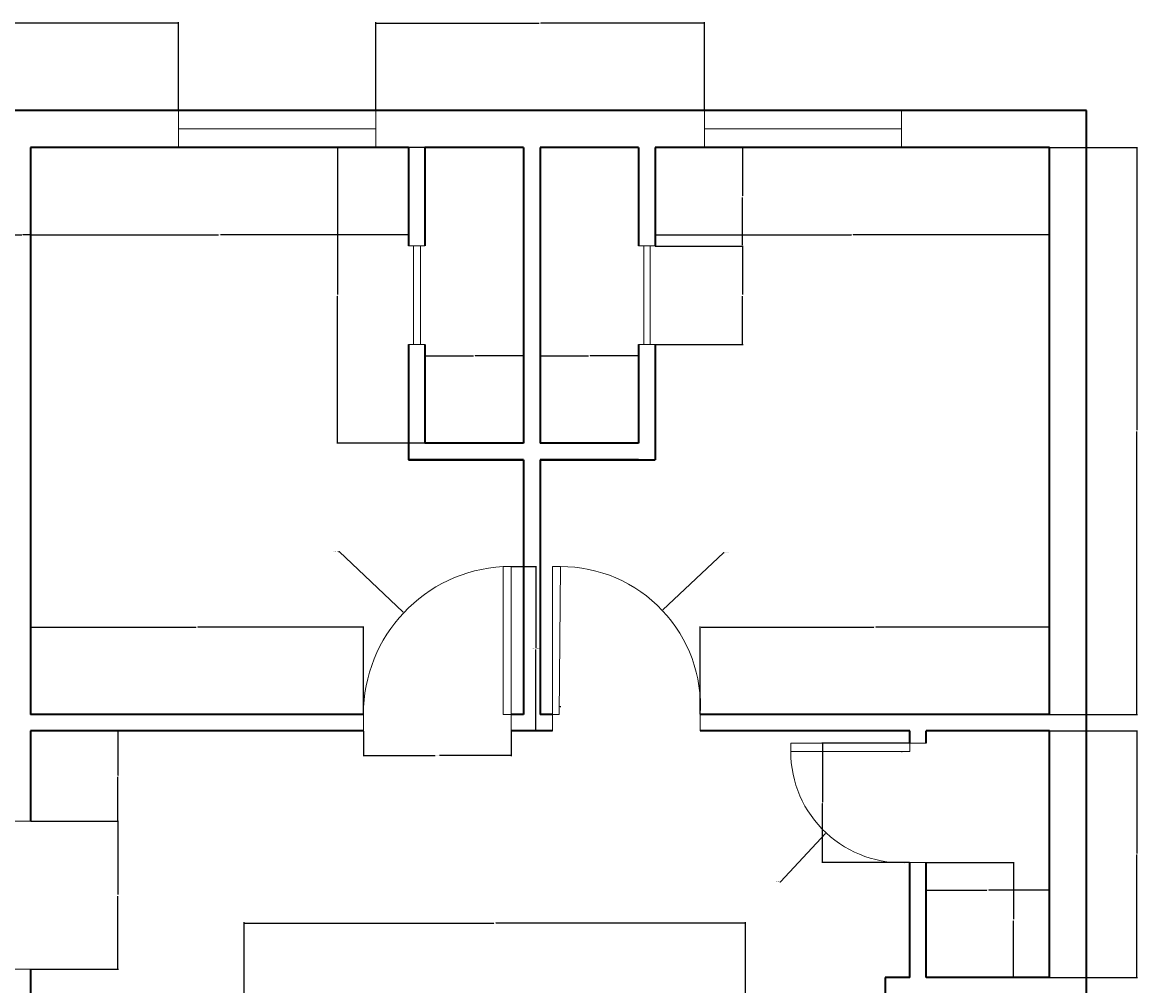
# Model space of a CAD drawing. Units: inches. Extents: x 2345 to 2781, y 2622 to 3032.
# Tile 3 of 3: x 2509 to 2781, y 2798 to 3032. Entities that reach past the tile are written whole.
import ezdxf

# ---------------------------------------------------------------- set-up
doc = ezdxf.new("R2010")
doc.units = ezdxf.units.IN
for name, color, linetype, lineweight in [('A-ANNO-DIMS', 2, 'Continuous', 18), ('A-DOOR', 3, 'Continuous', 18), ('A-GLAZ', 4, 'Continuous', 18), ('A-WALL', 7, 'Continuous', 35)]:
    doc.layers.add(name, color=color, linetype=linetype, lineweight=lineweight)
doc.styles.get("Standard").update_dxf_attribs({"font": 'arial.ttf'})
doc.dimstyles.get("Standard").update_dxf_attribs({"dimtxt": 0.18, "dimasz": 0.18, "dimexe": 0.18, "dimexo": 0.0625, "dimgap": 0.09, "dimtad": 0, "dimtih": 1, "dimtoh": 1, "dimdec": 4, "dimzin": 0, "dimdsep": 46, "dimtxsty": 'Standard', "dimcen": 0.09, "dimadec": 0, "dimazin": 0, "dimtfac": 1, "dimtdec": 4, "dimtofl": 0, "dimtmove": 0, "dimatfit": 3, "dimfxl": 1, "dimtolj": 1, "dimtzin": 0, "dimarcsym": 0})

# ---------------------------------------------------------------- blocks, each defined once
blk = doc.blocks.new('DOOR-36IN-SWING-A')
for p, q in [((36, 40), (34, 40)), ((34, 40), (34, 4)), ((36, 4), (36, 40)), ((0, 4), (0, 0)), ((34, 4), (36, 4)), ((36, 4), (36, 0))]:
    blk.add_line(p, q)
blk.add_arc((36.06, 4), 36.06, 93.2732, 180)
blk = doc.blocks.new('WIN-48IN')
for p, q in [((0, 0), (0, 9)), ((48, 0), (48, 9)), ((0, 4.5), (48, 4.5))]:
    blk.add_line(p, q)
blk = doc.blocks.new('*D4')
at = {"layer": 'A-ANNO-DIMS', "color": 0, "lineweight": -2, "transparency": 16777216}
for p, q in [((2628.33, 2899.8), (2634.45, 2899.8)), ((2634.27, 2899.62), (2634.27, 2879.99)), ((2634.27, 2859.98), (2634.27, 2879.62)), ((2628.33, 2859.8), (2634.45, 2859.8))]:
    blk.add_line(p, q, dxfattribs=at)
at = {"layer": 'A-ANNO-DIMS', "color": 0, "transparency": 16777216}
for points in [[(2634.24, 2899.62), (2634.3, 2899.62), (2634.27, 2899.8)], [(2634.24, 2859.98), (2634.3, 2859.98), (2634.27, 2859.8)]]:
    blk.add_solid(points, dxfattribs=at)
at = {"layer": 'Defpoints', "color": 0, "transparency": 16777216}
for p in [(2628.27, 2899.8), (2634.27, 2899.8), (2628.27, 2859.8)]:
    blk.add_point(p, dxfattribs=at)
at = {"layer": 'A-ANNO-DIMS', "color": 0, "transparency": 16777216, "insert": (2634.27, 2879.8), "char_height": 0.18, "attachment_point": 5}
blk.add_mtext('\\A1;DOOR A 40 TYP.', dxfattribs=at)
blk = doc.blocks.new('*D5')
at = {"layer": 'A-ANNO-DIMS', "color": 0, "lineweight": -2, "transparency": 16777216}
for p, q in [((2592.27, 2859.74), (2592.27, 2853.62)), ((2628.27, 2859.74), (2628.27, 2853.62)), ((2592.45, 2853.8), (2609.74, 2853.8)), ((2628.09, 2853.8), (2610.8, 2853.8))]:
    blk.add_line(p, q, dxfattribs=at)
at = {"layer": 'A-ANNO-DIMS', "color": 0, "transparency": 16777216}
for points in [[(2592.45, 2853.83), (2592.45, 2853.77), (2592.27, 2853.8)], [(2628.09, 2853.83), (2628.09, 2853.77), (2628.27, 2853.8)]]:
    blk.add_solid(points, dxfattribs=at)
at = {"layer": 'Defpoints', "color": 0, "transparency": 16777216}
for p in [(2592.27, 2859.8), (2628.27, 2859.8), (2628.27, 2853.8)]:
    blk.add_point(p, dxfattribs=at)
at = {"layer": 'A-ANNO-DIMS', "color": 0, "transparency": 16777216, "insert": (2610.27, 2853.8), "char_height": 0.18, "attachment_point": 5}
blk.add_mtext('\\A1;36 TYP.', dxfattribs=at)
blk = doc.blocks.new('*D13')
at = {"layer": 'A-ANNO-DIMS', "color": 0, "lineweight": -2, "transparency": 16777216}
for p, q in [((2459.27, 3010.87), (2459.27, 3032.23)), ((2547.27, 3010.87), (2547.27, 3032.23)), ((2459.45, 3032.05), (2503.05, 3032.05)), ((2547.09, 3032.05), (2503.49, 3032.05))]:
    blk.add_line(p, q, dxfattribs=at)
at = {"layer": 'A-ANNO-DIMS', "color": 0, "transparency": 16777216}
for points in [[(2459.45, 3032.08), (2459.45, 3032.02), (2459.27, 3032.05)], [(2547.09, 3032.08), (2547.09, 3032.02), (2547.27, 3032.05)]]:
    blk.add_solid(points, dxfattribs=at)
at = {"layer": 'Defpoints', "color": 0, "transparency": 16777216}
for p in [(2547.27, 3032.05), (2459.27, 3010.8), (2547.27, 3010.8)]:
    blk.add_point(p, dxfattribs=at)
at = {"layer": 'A-ANNO-DIMS', "color": 0, "transparency": 16777216, "insert": (2503.27, 3032.05), "char_height": 0.18, "attachment_point": 5}
blk.add_mtext('\\A1;88', dxfattribs=at)
blk = doc.blocks.new('*D14')
at = {"layer": 'A-ANNO-DIMS', "color": 0, "lineweight": -2, "transparency": 16777216}
for p, q in [((2595.27, 3010.87), (2595.27, 3032.23)), ((2675.27, 3010.87), (2675.27, 3032.23)), ((2595.45, 3032.05), (2635.05, 3032.05)), ((2675.09, 3032.05), (2635.49, 3032.05))]:
    blk.add_line(p, q, dxfattribs=at)
at = {"layer": 'A-ANNO-DIMS', "color": 0, "transparency": 16777216}
for points in [[(2595.45, 3032.08), (2595.45, 3032.02), (2595.27, 3032.05)], [(2675.09, 3032.08), (2675.09, 3032.02), (2675.27, 3032.05)]]:
    blk.add_solid(points, dxfattribs=at)
at = {"layer": 'Defpoints', "color": 0, "transparency": 16777216}
for p in [(2675.27, 3032.05), (2595.27, 3010.8), (2675.27, 3010.8)]:
    blk.add_point(p, dxfattribs=at)
at = {"layer": 'A-ANNO-DIMS', "color": 0, "transparency": 16777216, "insert": (2635.27, 3032.05), "char_height": 0.18, "attachment_point": 5}
blk.add_mtext('\\A1;80', dxfattribs=at)
blk = doc.blocks.new('*D16')
at = {"layer": 'A-ANNO-DIMS', "color": 0, "lineweight": -2, "transparency": 16777216}
for p, q in [((2507.27, 3001.74), (2507.27, 2980.37)), ((2511.27, 3001.74), (2511.27, 2980.37)), ((2507.45, 2980.55), (2509.12, 2980.55)), ((2511.09, 2980.55), (2509.42, 2980.55))]:
    blk.add_line(p, q, dxfattribs=at)
at = {"layer": 'A-ANNO-DIMS', "color": 0, "transparency": 16777216}
for points in [[(2507.45, 2980.58), (2507.45, 2980.52), (2507.27, 2980.55)], [(2511.09, 2980.58), (2511.09, 2980.52), (2511.27, 2980.55)]]:
    blk.add_solid(points, dxfattribs=at)
at = {"layer": 'Defpoints', "color": 0, "transparency": 16777216}
for p in [(2507.27, 3001.8), (2511.27, 3001.8), (2507.27, 2980.55)]:
    blk.add_point(p, dxfattribs=at)
at = {"layer": 'A-ANNO-DIMS', "color": 0, "transparency": 16777216, "insert": (2509.27, 2980.55), "char_height": 0.18, "attachment_point": 5}
blk.add_mtext('\\A1;4', dxfattribs=at)
blk = doc.blocks.new('*D17')
at = {"layer": 'A-ANNO-DIMS', "color": 0, "lineweight": -2, "transparency": 16777216}
for p, q in [((2511.27, 3001.74), (2511.27, 2980.37)), ((2603.27, 3001.74), (2603.27, 2980.37)), ((2511.45, 2980.55), (2557.05, 2980.55)), ((2603.09, 2980.55), (2557.49, 2980.55))]:
    blk.add_line(p, q, dxfattribs=at)
at = {"layer": 'A-ANNO-DIMS', "color": 0, "transparency": 16777216}
for points in [[(2511.45, 2980.58), (2511.45, 2980.52), (2511.27, 2980.55)], [(2603.09, 2980.58), (2603.09, 2980.52), (2603.27, 2980.55)]]:
    blk.add_solid(points, dxfattribs=at)
at = {"layer": 'Defpoints', "color": 0, "transparency": 16777216}
for p in [(2511.27, 3001.8), (2603.27, 3001.8), (2511.27, 2980.55)]:
    blk.add_point(p, dxfattribs=at)
at = {"layer": 'A-ANNO-DIMS', "color": 0, "transparency": 16777216, "insert": (2557.27, 2980.55), "char_height": 0.18, "attachment_point": 5}
blk.add_mtext('\\A1;92', dxfattribs=at)
blk = doc.blocks.new('*D18')
at = {"layer": 'A-ANNO-DIMS', "color": 0, "lineweight": -2, "transparency": 16777216}
for p, q in [((2663.27, 3001.74), (2663.27, 2980.37)), ((2759.27, 3001.74), (2759.27, 2980.37)), ((2663.45, 2980.55), (2711.05, 2980.55)), ((2759.09, 2980.55), (2711.49, 2980.55))]:
    blk.add_line(p, q, dxfattribs=at)
at = {"layer": 'A-ANNO-DIMS', "color": 0, "transparency": 16777216}
for points in [[(2663.45, 2980.58), (2663.45, 2980.52), (2663.27, 2980.55)], [(2759.09, 2980.58), (2759.09, 2980.52), (2759.27, 2980.55)]]:
    blk.add_solid(points, dxfattribs=at)
at = {"layer": 'Defpoints', "color": 0, "transparency": 16777216}
for p in [(2663.27, 3001.8), (2759.27, 3001.8), (2663.27, 2980.55)]:
    blk.add_point(p, dxfattribs=at)
at = {"layer": 'A-ANNO-DIMS', "color": 0, "transparency": 16777216, "insert": (2711.27, 2980.55), "char_height": 0.18, "attachment_point": 5}
blk.add_mtext('\\A1;96', dxfattribs=at)
blk = doc.blocks.new('*D19')
at = {"layer": 'A-ANNO-DIMS', "color": 0, "lineweight": -2, "transparency": 16777216}
for p, q in [((2607.27, 2929.87), (2607.27, 2951.23)), ((2607.45, 2951.05), (2619.05, 2951.05)), ((2631.09, 2951.05), (2619.49, 2951.05)), ((2631.27, 2929.87), (2631.27, 2951.23))]:
    blk.add_line(p, q, dxfattribs=at)
at = {"layer": 'A-ANNO-DIMS', "color": 0, "transparency": 16777216}
for points in [[(2607.45, 2951.08), (2607.45, 2951.02), (2607.27, 2951.05)], [(2631.09, 2951.08), (2631.09, 2951.02), (2631.27, 2951.05)]]:
    blk.add_solid(points, dxfattribs=at)
at = {"layer": 'Defpoints', "color": 0, "transparency": 16777216}
for p in [(2631.27, 2951.05), (2607.27, 2929.8), (2631.27, 2929.8)]:
    blk.add_point(p, dxfattribs=at)
at = {"layer": 'A-ANNO-DIMS', "color": 0, "transparency": 16777216, "insert": (2619.27, 2951.05), "char_height": 0.18, "attachment_point": 5}
blk.add_mtext('\\A1;24', dxfattribs=at)
blk = doc.blocks.new('*D20')
at = {"layer": 'A-ANNO-DIMS', "color": 0, "lineweight": -2, "transparency": 16777216}
for p, q in [((2635.27, 2929.87), (2635.27, 2951.23)), ((2635.45, 2951.05), (2647.05, 2951.05)), ((2659.09, 2951.05), (2647.49, 2951.05)), ((2659.27, 2929.87), (2659.27, 2951.23))]:
    blk.add_line(p, q, dxfattribs=at)
at = {"layer": 'A-ANNO-DIMS', "color": 0, "transparency": 16777216}
for points in [[(2635.45, 2951.08), (2635.45, 2951.02), (2635.27, 2951.05)], [(2659.09, 2951.08), (2659.09, 2951.02), (2659.27, 2951.05)]]:
    blk.add_solid(points, dxfattribs=at)
at = {"layer": 'Defpoints', "color": 0, "transparency": 16777216}
for p in [(2659.27, 2951.05), (2635.27, 2929.8), (2659.27, 2929.8)]:
    blk.add_point(p, dxfattribs=at)
at = {"layer": 'A-ANNO-DIMS', "color": 0, "transparency": 16777216, "insert": (2647.27, 2951.05), "char_height": 0.18, "attachment_point": 5}
blk.add_mtext('\\A1;24', dxfattribs=at)
blk = doc.blocks.new('*D21')
at = {"layer": 'A-ANNO-DIMS', "color": 0, "lineweight": -2, "transparency": 16777216}
for p, q in [((2607.21, 3001.8), (2585.84, 3001.8)), ((2586.02, 3001.62), (2586.02, 2965.98)), ((2586.02, 2929.98), (2586.02, 2965.62)), ((2607.21, 2929.8), (2585.84, 2929.8))]:
    blk.add_line(p, q, dxfattribs=at)
at = {"layer": 'A-ANNO-DIMS', "color": 0, "transparency": 16777216}
for points in [[(2585.99, 3001.62), (2586.05, 3001.62), (2586.02, 3001.8)], [(2585.99, 2929.98), (2586.05, 2929.98), (2586.02, 2929.8)]]:
    blk.add_solid(points, dxfattribs=at)
at = {"layer": 'Defpoints', "color": 0, "transparency": 16777216}
for p in [(2586.02, 3001.8), (2607.27, 3001.8), (2607.27, 2929.8)]:
    blk.add_point(p, dxfattribs=at)
at = {"layer": 'A-ANNO-DIMS', "color": 0, "transparency": 16777216, "insert": (2586.02, 2965.8), "char_height": 0.18, "attachment_point": 5}
blk.add_mtext('\\A1;72', dxfattribs=at)
blk = doc.blocks.new('*D22')
at = {"layer": 'A-ANNO-DIMS', "color": 0, "lineweight": -2, "transparency": 16777216}
for p, q in [((2663.33, 3001.8), (2684.7, 3001.8)), ((2684.52, 3001.62), (2684.52, 2989.98)), ((2684.52, 2977.98), (2684.52, 2989.62)), ((2663.33, 2977.8), (2684.7, 2977.8))]:
    blk.add_line(p, q, dxfattribs=at)
at = {"layer": 'A-ANNO-DIMS', "color": 0, "transparency": 16777216}
for points in [[(2684.49, 3001.62), (2684.55, 3001.62), (2684.52, 3001.8)], [(2684.49, 2977.98), (2684.55, 2977.98), (2684.52, 2977.8)]]:
    blk.add_solid(points, dxfattribs=at)
at = {"layer": 'Defpoints', "color": 0, "transparency": 16777216}
for p in [(2663.27, 3001.8), (2663.27, 2977.8), (2684.52, 2977.8)]:
    blk.add_point(p, dxfattribs=at)
at = {"layer": 'A-ANNO-DIMS', "color": 0, "transparency": 16777216, "insert": (2684.52, 2989.8), "char_height": 0.18, "attachment_point": 5}
blk.add_mtext('\\A1;24', dxfattribs=at)
blk = doc.blocks.new('*D23')
at = {"layer": 'A-ANNO-DIMS', "color": 0, "lineweight": -2, "transparency": 16777216}
for p, q in [((2663.33, 2977.8), (2684.7, 2977.8)), ((2684.52, 2977.62), (2684.52, 2965.98)), ((2684.52, 2953.98), (2684.52, 2965.62)), ((2663.33, 2953.8), (2684.7, 2953.8))]:
    blk.add_line(p, q, dxfattribs=at)
at = {"layer": 'A-ANNO-DIMS', "color": 0, "transparency": 16777216}
for points in [[(2684.49, 2977.62), (2684.55, 2977.62), (2684.52, 2977.8)], [(2684.49, 2953.98), (2684.55, 2953.98), (2684.52, 2953.8)]]:
    blk.add_solid(points, dxfattribs=at)
at = {"layer": 'Defpoints', "color": 0, "transparency": 16777216}
for p in [(2663.27, 2977.8), (2663.27, 2953.8), (2684.52, 2953.8)]:
    blk.add_point(p, dxfattribs=at)
at = {"layer": 'A-ANNO-DIMS', "color": 0, "transparency": 16777216, "insert": (2684.52, 2965.8), "char_height": 0.18, "attachment_point": 5}
blk.add_mtext('\\A1;24', dxfattribs=at)
blk = doc.blocks.new('*D25')
at = {"layer": 'A-ANNO-DIMS', "color": 0, "lineweight": -2, "transparency": 16777216}
for p, q in [((2759.33, 3001.8), (2780.7, 3001.8)), ((2780.52, 3001.62), (2780.52, 2932.98)), ((2780.52, 2863.98), (2780.52, 2932.62)), ((2759.33, 2863.8), (2780.7, 2863.8))]:
    blk.add_line(p, q, dxfattribs=at)
at = {"layer": 'A-ANNO-DIMS', "color": 0, "transparency": 16777216}
for points in [[(2780.49, 3001.62), (2780.55, 3001.62), (2780.52, 3001.8)], [(2780.49, 2863.98), (2780.55, 2863.98), (2780.52, 2863.8)]]:
    blk.add_solid(points, dxfattribs=at)
at = {"layer": 'Defpoints', "color": 0, "transparency": 16777216}
for p in [(2759.27, 3001.8), (2759.27, 2863.8), (2780.52, 2863.8)]:
    blk.add_point(p, dxfattribs=at)
at = {"layer": 'A-ANNO-DIMS', "color": 0, "transparency": 16777216, "insert": (2780.52, 2932.8), "char_height": 0.18, "attachment_point": 5}
blk.add_mtext('\\A1;138', dxfattribs=at)
blk = doc.blocks.new('*D28')
at = {"layer": 'A-ANNO-DIMS', "color": 0, "lineweight": -2, "transparency": 16777216}
for p, q in [((2511.33, 2837.8), (2532.7, 2837.8)), ((2532.52, 2837.62), (2532.52, 2819.98)), ((2532.52, 2801.98), (2532.52, 2819.62)), ((2511.33, 2801.8), (2532.7, 2801.8))]:
    blk.add_line(p, q, dxfattribs=at)
at = {"layer": 'A-ANNO-DIMS', "color": 0, "transparency": 16777216}
for points in [[(2532.49, 2837.62), (2532.55, 2837.62), (2532.52, 2837.8)], [(2532.49, 2801.98), (2532.55, 2801.98), (2532.52, 2801.8)]]:
    blk.add_solid(points, dxfattribs=at)
at = {"layer": 'Defpoints', "color": 0, "transparency": 16777216}
for p in [(2511.27, 2837.8), (2511.27, 2801.8), (2532.52, 2801.8)]:
    blk.add_point(p, dxfattribs=at)
at = {"layer": 'A-ANNO-DIMS', "color": 0, "transparency": 16777216, "insert": (2532.52, 2819.8), "char_height": 0.18, "attachment_point": 5}
blk.add_mtext('\\A1;36', dxfattribs=at)
blk = doc.blocks.new('*D29')
at = {"layer": 'A-ANNO-DIMS', "color": 0, "lineweight": -2, "transparency": 16777216}
for p, q in [((2511.33, 2859.8), (2532.7, 2859.8)), ((2532.52, 2859.62), (2532.52, 2848.98)), ((2532.52, 2837.98), (2532.52, 2848.62)), ((2511.33, 2837.8), (2532.7, 2837.8))]:
    blk.add_line(p, q, dxfattribs=at)
at = {"layer": 'A-ANNO-DIMS', "color": 0, "transparency": 16777216}
for points in [[(2532.49, 2859.62), (2532.55, 2859.62), (2532.52, 2859.8)], [(2532.49, 2837.98), (2532.55, 2837.98), (2532.52, 2837.8)]]:
    blk.add_solid(points, dxfattribs=at)
at = {"layer": 'Defpoints', "color": 0, "transparency": 16777216}
for p in [(2511.27, 2859.8), (2511.27, 2837.8), (2532.52, 2837.8)]:
    blk.add_point(p, dxfattribs=at)
at = {"layer": 'A-ANNO-DIMS', "color": 0, "transparency": 16777216, "insert": (2532.52, 2848.8), "char_height": 0.18, "attachment_point": 5}
blk.add_mtext('\\A1;22', dxfattribs=at)
blk = doc.blocks.new('*D30')
at = {"layer": 'A-ANNO-DIMS', "color": 0, "lineweight": -2, "transparency": 16777216}
for p, q in [((2511.27, 2863.87), (2511.27, 2885.23)), ((2511.45, 2885.05), (2551.57, 2885.05)), ((2592.09, 2885.05), (2551.97, 2885.05)), ((2592.27, 2863.87), (2592.27, 2885.23))]:
    blk.add_line(p, q, dxfattribs=at)
at = {"layer": 'A-ANNO-DIMS', "color": 0, "transparency": 16777216}
for points in [[(2511.45, 2885.08), (2511.45, 2885.02), (2511.27, 2885.05)], [(2592.09, 2885.08), (2592.09, 2885.02), (2592.27, 2885.05)]]:
    blk.add_solid(points, dxfattribs=at)
at = {"layer": 'Defpoints', "color": 0, "transparency": 16777216}
for p in [(2592.27, 2885.05), (2511.27, 2863.8), (2592.27, 2863.8)]:
    blk.add_point(p, dxfattribs=at)
at = {"layer": 'A-ANNO-DIMS', "color": 0, "transparency": 16777216, "insert": (2551.77, 2885.05), "char_height": 0.18, "attachment_point": 5}
blk.add_mtext('\\A1;81', dxfattribs=at)
blk = doc.blocks.new('*D31')
at = {"layer": 'A-ANNO-DIMS', "color": 0, "lineweight": -2, "transparency": 16777216}
for p, q in [((2674.27, 2863.87), (2674.27, 2885.23)), ((2674.45, 2885.05), (2716.55, 2885.05)), ((2759.09, 2885.05), (2716.99, 2885.05)), ((2759.27, 2863.87), (2759.27, 2885.23))]:
    blk.add_line(p, q, dxfattribs=at)
at = {"layer": 'A-ANNO-DIMS', "color": 0, "transparency": 16777216}
for points in [[(2674.45, 2885.08), (2674.45, 2885.02), (2674.27, 2885.05)], [(2759.09, 2885.08), (2759.09, 2885.02), (2759.27, 2885.05)]]:
    blk.add_solid(points, dxfattribs=at)
at = {"layer": 'Defpoints', "color": 0, "transparency": 16777216}
for p in [(2759.27, 2885.05), (2674.27, 2863.8), (2759.27, 2863.8)]:
    blk.add_point(p, dxfattribs=at)
at = {"layer": 'A-ANNO-DIMS', "color": 0, "transparency": 16777216, "insert": (2716.77, 2885.05), "char_height": 0.18, "attachment_point": 5}
blk.add_mtext('\\A1;85', dxfattribs=at)
blk = doc.blocks.new('*D39')
at = {"layer": 'A-ANNO-DIMS', "color": 0, "lineweight": -2, "transparency": 16777216}
for p, q in [((2563.27, 2791.87), (2563.27, 2813.23)), ((2563.45, 2813.05), (2623.99, 2813.05)), ((2685.09, 2813.05), (2624.55, 2813.05)), ((2685.27, 2791.87), (2685.27, 2813.23))]:
    blk.add_line(p, q, dxfattribs=at)
at = {"layer": 'A-ANNO-DIMS', "color": 0, "transparency": 16777216}
for points in [[(2563.45, 2813.08), (2563.45, 2813.02), (2563.27, 2813.05)], [(2685.09, 2813.08), (2685.09, 2813.02), (2685.27, 2813.05)]]:
    blk.add_solid(points, dxfattribs=at)
at = {"layer": 'Defpoints', "color": 0, "transparency": 16777216}
for p in [(2685.27, 2813.05), (2563.27, 2791.8), (2685.27, 2791.8)]:
    blk.add_point(p, dxfattribs=at)
at = {"layer": 'A-ANNO-DIMS', "color": 0, "transparency": 16777216, "insert": (2624.27, 2813.05), "char_height": 0.18, "attachment_point": 5}
blk.add_mtext('\\A1;122', dxfattribs=at)
blk = doc.blocks.new('*D41')
at = {"layer": 'A-ANNO-DIMS', "color": 0, "lineweight": -2, "transparency": 16777216}
for p, q in [((2729.27, 2799.87), (2729.27, 2821.23)), ((2729.45, 2821.05), (2744.05, 2821.05)), ((2759.09, 2821.05), (2744.49, 2821.05)), ((2759.27, 2799.87), (2759.27, 2821.23))]:
    blk.add_line(p, q, dxfattribs=at)
at = {"layer": 'A-ANNO-DIMS', "color": 0, "transparency": 16777216}
for points in [[(2729.45, 2821.08), (2729.45, 2821.02), (2729.27, 2821.05)], [(2759.09, 2821.08), (2759.09, 2821.02), (2759.27, 2821.05)]]:
    blk.add_solid(points, dxfattribs=at)
at = {"layer": 'Defpoints', "color": 0, "transparency": 16777216}
for p in [(2759.27, 2821.05), (2729.27, 2799.8), (2759.27, 2799.8)]:
    blk.add_point(p, dxfattribs=at)
at = {"layer": 'A-ANNO-DIMS', "color": 0, "transparency": 16777216, "insert": (2744.27, 2821.05), "char_height": 0.18, "attachment_point": 5}
blk.add_mtext('\\A1;30', dxfattribs=at)
blk = doc.blocks.new('*D42')
at = {"layer": 'A-ANNO-DIMS', "color": 0, "lineweight": -2, "transparency": 16777216}
for p, q in [((2759.33, 2859.8), (2780.7, 2859.8)), ((2780.52, 2859.62), (2780.52, 2829.98)), ((2780.52, 2799.98), (2780.52, 2829.62)), ((2759.33, 2799.8), (2780.7, 2799.8))]:
    blk.add_line(p, q, dxfattribs=at)
at = {"layer": 'A-ANNO-DIMS', "color": 0, "transparency": 16777216}
for points in [[(2780.49, 2859.62), (2780.55, 2859.62), (2780.52, 2859.8)], [(2780.49, 2799.98), (2780.55, 2799.98), (2780.52, 2799.8)]]:
    blk.add_solid(points, dxfattribs=at)
at = {"layer": 'Defpoints', "color": 0, "transparency": 16777216}
for p in [(2759.27, 2859.8), (2759.27, 2799.8), (2780.52, 2799.8)]:
    blk.add_point(p, dxfattribs=at)
at = {"layer": 'A-ANNO-DIMS', "color": 0, "transparency": 16777216, "insert": (2780.52, 2829.8), "char_height": 0.18, "attachment_point": 5}
blk.add_mtext('\\A1;60', dxfattribs=at)
blk = doc.blocks.new('*D43')
at = {"layer": 'A-ANNO-DIMS', "color": 0, "lineweight": -2, "transparency": 16777216}
for p, q in [((2725.21, 2856.8), (2703.84, 2856.8)), ((2704.02, 2856.62), (2704.02, 2842.48)), ((2704.02, 2827.98), (2704.02, 2842.12)), ((2725.21, 2827.8), (2703.84, 2827.8))]:
    blk.add_line(p, q, dxfattribs=at)
at = {"layer": 'A-ANNO-DIMS', "color": 0, "transparency": 16777216}
for points in [[(2703.99, 2856.62), (2704.05, 2856.62), (2704.02, 2856.8)], [(2703.99, 2827.98), (2704.05, 2827.98), (2704.02, 2827.8)]]:
    blk.add_solid(points, dxfattribs=at)
at = {"layer": 'Defpoints', "color": 0, "transparency": 16777216}
for p in [(2704.02, 2856.8), (2725.27, 2856.8), (2725.27, 2827.8)]:
    blk.add_point(p, dxfattribs=at)
at = {"layer": 'A-ANNO-DIMS', "color": 0, "transparency": 16777216, "insert": (2704.02, 2842.3), "char_height": 0.18, "attachment_point": 5}
blk.add_mtext('\\A1;29', dxfattribs=at)
blk = doc.blocks.new('*D44')
at = {"layer": 'A-ANNO-DIMS', "color": 0, "lineweight": -2, "transparency": 16777216}
for p, q in [((2729.33, 2827.8), (2750.7, 2827.8)), ((2750.52, 2827.62), (2750.52, 2813.98)), ((2750.52, 2799.98), (2750.52, 2813.62)), ((2729.33, 2799.8), (2750.7, 2799.8))]:
    blk.add_line(p, q, dxfattribs=at)
at = {"layer": 'A-ANNO-DIMS', "color": 0, "transparency": 16777216}
for points in [[(2750.49, 2827.62), (2750.55, 2827.62), (2750.52, 2827.8)], [(2750.49, 2799.98), (2750.55, 2799.98), (2750.52, 2799.8)]]:
    blk.add_solid(points, dxfattribs=at)
at = {"layer": 'Defpoints', "color": 0, "transparency": 16777216}
for p in [(2729.27, 2827.8), (2729.27, 2799.8), (2750.52, 2799.8)]:
    blk.add_point(p, dxfattribs=at)
at = {"layer": 'A-ANNO-DIMS', "color": 0, "transparency": 16777216, "insert": (2750.52, 2813.8), "char_height": 0.18, "attachment_point": 5}
blk.add_mtext('\\A1;28', dxfattribs=at)
blk = doc.blocks.new('*D65')
at = {"layer": 'A-ANNO-DIMS', "color": 0, "lineweight": -2, "transparency": 16777216}
for p, q in [((2586.21, 2903.42), (2586.39, 2903.42)), ((2586.39, 2903.42), (2601.98, 2888.69)), ((2628.33, 2863.71), (2628.33, 2863.89)), ((2628.24, 2863.8), (2628.42, 2863.8))]:
    blk.add_line(p, q, dxfattribs=at)
at = {"layer": 'A-ANNO-DIMS', "color": 0, "transparency": 16777216}
blk.add_solid([(2602.01, 2888.71), (2601.96, 2888.66), (2602.12, 2888.56)], dxfattribs=at)
at = {"layer": 'Defpoints', "color": 0, "transparency": 16777216}
for p in [(2602.12, 2888.56), (2628.33, 2863.8)]:
    blk.add_point(p, dxfattribs=at)
at = {"layer": 'A-ANNO-DIMS', "color": 0, "transparency": 16777216, "insert": (2585.53, 2903.42), "char_height": 0.18, "attachment_point": 5}
blk.add_mtext('\\A1;2X R36.06', dxfattribs=at)
blk = doc.blocks.new('*D66')
at = {"layer": 'A-ANNO-DIMS', "color": 0, "lineweight": -2, "transparency": 16777216}
for p, q in [((2679.89, 2903.16), (2665.16, 2889.25)), ((2680.07, 2903.16), (2679.89, 2903.16)), ((2640.18, 2865.75), (2640.36, 2865.75)), ((2640.27, 2865.66), (2640.27, 2865.84))]:
    blk.add_line(p, q, dxfattribs=at)
at = {"layer": 'A-ANNO-DIMS', "color": 0, "transparency": 16777216}
blk.add_solid([(2665.14, 2889.28), (2665.18, 2889.23), (2665.03, 2889.13)], dxfattribs=at)
at = {"layer": 'Defpoints', "color": 0, "transparency": 16777216}
for p in [(2665.03, 2889.13), (2640.27, 2865.75)]:
    blk.add_point(p, dxfattribs=at)
at = {"layer": 'A-ANNO-DIMS', "color": 0, "transparency": 16777216, "insert": (2680.81, 2903.16), "char_height": 0.18, "attachment_point": 5}
blk.add_mtext('\\A1;3X R34.056', dxfattribs=at)
blk = doc.blocks.new('*D69')
at = {"layer": 'A-ANNO-DIMS', "color": 0, "lineweight": -2, "transparency": 16777216}
for p, q in [((2723.25, 2854.8), (2723.43, 2854.8)), ((2723.34, 2854.71), (2723.34, 2854.89)), ((2693.83, 2823.1), (2704.77, 2834.86)), ((2693.65, 2823.1), (2693.83, 2823.1))]:
    blk.add_line(p, q, dxfattribs=at)
at = {"layer": 'A-ANNO-DIMS', "color": 0, "transparency": 16777216}
blk.add_solid([(2704.75, 2834.88), (2704.8, 2834.84), (2704.9, 2834.99)], dxfattribs=at)
at = {"layer": 'Defpoints', "color": 0, "transparency": 16777216}
for p in [(2723.34, 2854.8), (2704.9, 2834.99)]:
    blk.add_point(p, dxfattribs=at)
at = {"layer": 'A-ANNO-DIMS', "color": 0, "transparency": 16777216, "insert": (2693.17, 2823.1), "char_height": 0.18, "attachment_point": 5}
blk.add_mtext('\\A1;R27.07', dxfattribs=at)

msp = doc.modelspace()

# ---------------------------------------------------------------- linework, layer by layer
at = {"layer": 'A-DOOR'}
for p, q in [((2603.2719, 2977.8029), (2607.2719, 2977.8029)), ((2604.4427, 2977.8029), (2604.4427, 2953.8029)), ((2606.1611, 2977.8029), (2606.1611, 2953.8029)), ((2659.2719, 2977.8029), (2663.2719, 2977.8029)), ((2660.5235, 2977.8029), (2660.5235, 2953.8029)), ((2662.0619, 2977.8029), (2662.0619, 2953.8029)), ((2603.2719, 2953.8029), (2607.2719, 2953.8029)), ((2659.2719, 2953.8029), (2663.2719, 2953.8029)), ((2638.2719, 2863.8029), (2638.2719, 2899.803)), ((2638.2719, 2899.803), (2640.2719, 2899.803)), ((2640.2719, 2899.803), (2639.9286, 2863.8029)), ((2638.2719, 2863.8029), (2638.2719, 2859.8029)), ((2639.9286, 2863.8029), (2638.2719, 2863.8029)), ((2674.2719, 2863.8029), (2674.2719, 2859.8029)), ((2725.2719, 2856.8029), (2696.2719, 2856.8029)), ((2696.2719, 2856.8029), (2696.2719, 2854.8029)), ((2725.2719, 2856.8029), (2729.2719, 2856.8029)), ((2725.2719, 2854.8029), (2725.2719, 2856.8029)), ((2696.2719, 2854.8029), (2725.2719, 2854.8029)), ((2507.2719, 2837.8029), (2511.2719, 2837.8029)), ((2725.2719, 2827.8029), (2729.2719, 2827.8029)), ((2507.2719, 2801.8029), (2511.2719, 2801.8029))]:
    msp.add_line(p, q, dxfattribs=at)
for centre, radius, start, end in [((2640.2719, 2865.7474), 34.0556, 356.726846, 90), ((2723.3409, 2854.8029), 27.069, 180, 274.090817)]:
    msp.add_arc(centre, radius, start, end, dxfattribs=at)
at = {"layer": 'A-WALL'}
for p, q in [((2768.2719, 3010.8029), (2366.2719, 3010.8029)), ((2768.2719, 2643.803), (2768.2719, 3010.8029)), ((2511.2719, 3001.8029), (2511.2719, 2863.8029)), ((2603.2719, 3001.8029), (2511.2719, 3001.8029)), ((2603.2719, 3001.8029), (2603.2719, 2977.8029)), ((2631.2719, 3001.8029), (2607.2719, 3001.8029)), ((2607.2719, 3001.8029), (2607.2719, 2977.8029)), ((2631.2719, 3001.8029), (2631.2719, 2929.8029)), ((2635.2719, 3001.8029), (2635.2719, 2929.8029)), ((2659.2719, 3001.8029), (2635.2719, 3001.8029)), ((2659.2719, 3001.8029), (2659.2719, 2977.8029)), ((2759.2719, 3001.8029), (2663.2719, 3001.8029)), ((2663.2719, 3001.8029), (2663.2719, 2977.8029)), ((2759.2719, 2863.8029), (2759.2719, 3001.8029)), ((2603.2719, 2953.8029), (2603.2719, 2925.803)), ((2607.2719, 2953.8029), (2607.2719, 2929.8029)), ((2659.2719, 2953.8029), (2659.2719, 2929.8029)), ((2663.2719, 2953.8029), (2663.2719, 2925.803)), ((2631.2719, 2929.8029), (2607.2719, 2929.8029)), ((2659.2719, 2929.8029), (2635.2719, 2929.8029)), ((2607.2719, 2925.803), (2603.2719, 2925.803)), ((2603.2719, 2925.803), (2631.2719, 2925.803)), ((2631.2719, 2925.803), (2607.2719, 2925.803)), ((2631.2719, 2925.803), (2631.2719, 2863.8029)), ((2659.2719, 2925.803), (2635.2719, 2925.803)), ((2635.2719, 2925.803), (2663.2719, 2925.803)), ((2635.2719, 2925.803), (2635.2719, 2863.8029)), ((2592.2719, 2863.8029), (2511.2719, 2863.8029)), ((2631.2719, 2863.8029), (2628.2719, 2863.8029)), ((2638.2719, 2863.8029), (2635.2719, 2863.8029)), ((2759.2719, 2863.8029), (2674.2719, 2863.8029)), ((2511.2719, 2859.8029), (2511.2719, 2837.8029)), ((2592.2719, 2859.8029), (2511.2719, 2859.8029)), ((2638.2719, 2859.8029), (2628.2719, 2859.8029)), ((2725.2719, 2859.8029), (2674.2719, 2859.8029)), ((2725.2719, 2856.8029), (2725.2719, 2859.8029)), ((2759.2719, 2859.8029), (2729.2719, 2859.8029)), ((2729.2719, 2856.8029), (2729.2719, 2859.8029)), ((2759.2719, 2799.8029), (2759.2719, 2859.8029)), ((2725.2719, 2799.8029), (2725.2719, 2827.8029)), ((2729.2719, 2799.8029), (2729.2719, 2827.8029)), ((2511.2719, 2801.8029), (2511.2719, 2739.803)), ((2725.2719, 2799.8029), (2719.2719, 2799.8029)), ((2719.2719, 2799.8029), (2719.2719, 2795.803)), ((2759.2719, 2799.8029), (2729.2719, 2799.8029))]:
    msp.add_line(p, q, dxfattribs=at)

# ---------------------------------------------------------------- block references
at = {"layer": 'A-DOOR'}
msp.add_blockref('DOOR-36IN-SWING-A', (2592.272, 2859.803), dxfattribs=at)
at = {"layer": 'A-GLAZ'}
for p in [(2547.272, 3001.803), (2675.272, 3001.803)]:
    msp.add_blockref('WIN-48IN', p, dxfattribs=at)

# ---------------------------------------------------------------- dimensions: what is measured, and where the dimension line sits
at = {"layer": 'A-ANNO-DIMS'}
for base, p1, p2, picture, middle in [((2547.2719, 3032.0529), (2459.2719, 3010.8029), (2547.2719, 3010.8029), '*D13', (2503.2719, 3032.0529)), ((2675.2719, 3032.0529), (2595.2719, 3010.8029), (2675.2719, 3010.8029), '*D14', (2635.2719, 3032.0529)), ((2631.2719, 2951.0529), (2607.2719, 2929.8029), (2631.2719, 2929.8029), '*D19', (2619.2719, 2951.0529)), ((2659.2719, 2951.0529), (2635.2719, 2929.8029), (2659.2719, 2929.8029), '*D20', (2647.2719, 2951.0529)), ((2592.2719, 2885.0529), (2511.2719, 2863.8029), (2592.2719, 2863.8029), '*D30', (2551.7719, 2885.0529)), ((2759.2719, 2821.0529), (2729.2719, 2799.8029), (2759.2719, 2799.8029), '*D41', (2744.2719, 2821.0529)), ((2685.2719, 2813.0529), (2563.2719, 2791.8029), (2685.2719, 2791.8029), '*D39', (2624.2719, 2813.0529))]:
    dim = msp.add_linear_dim(base=base, p1=p1, p2=p2, dimstyle='Standard', override={"dimdec": 0, "dimlfac": 1, "dimrnd": 0, "dimzin": 0, "dimdsep": 46, "dimlunit": 2}, dxfattribs=at)
    dim.commit()
    dim.dimension.update_dxf_attribs({"geometry": picture, "text_midpoint": middle})
for base, p1, p2, angle, picture, middle in [((2507.2719, 2980.5529), (2511.2719, 3001.8029), (2507.2719, 3001.8029), 180, '*D16', (2509.2719, 2980.5529)), ((2511.2719, 2980.5529), (2603.2719, 3001.8029), (2511.2719, 3001.8029), 180, '*D17', (2557.2719, 2980.5529)), ((2586.0219, 3001.8029), (2607.2719, 2929.8029), (2607.2719, 3001.8029), 90, '*D21', (2586.0219, 2965.8029)), ((2684.5219, 2977.8029), (2663.2719, 3001.8029), (2663.2719, 2977.8029), 270, '*D22', (2684.5219, 2989.8029)), ((2663.2719, 2980.5529), (2759.2719, 3001.8029), (2663.2719, 3001.8029), 180, '*D18', (2711.2719, 2980.5529)), ((2780.5219, 2863.8029), (2759.2719, 3001.8029), (2759.2719, 2863.8029), 270, '*D25', (2780.5219, 2932.8029)), ((2684.5219, 2953.8029), (2663.2719, 2977.8029), (2663.2719, 2953.8029), 270, '*D23', (2684.5219, 2965.8029)), ((2759.2719, 2885.0529), (2674.2719, 2863.8029), (2759.2719, 2863.8029), 0, '*D31', (2716.7719, 2885.0529)), ((2532.5219, 2837.8029), (2511.2719, 2859.8029), (2511.2719, 2837.8029), 270, '*D29', (2532.5219, 2848.8029)), ((2780.5219, 2799.8029), (2759.2719, 2859.8029), (2759.2719, 2799.8029), 270, '*D42', (2780.5219, 2829.8029)), ((2704.0219, 2856.8029), (2725.2719, 2827.8029), (2725.2719, 2856.8029), 90, '*D43', (2704.0219, 2842.3029)), ((2532.5219, 2801.8029), (2511.2719, 2837.8029), (2511.2719, 2801.8029), 270, '*D28', (2532.5219, 2819.8029)), ((2750.5219, 2799.8029), (2729.2719, 2827.8029), (2729.2719, 2799.8029), 270, '*D44', (2750.5219, 2813.8029))]:
    dim = msp.add_linear_dim(base=base, p1=p1, p2=p2, angle=angle, dimstyle='Standard', override={"dimdec": 0, "dimlfac": 1, "dimrnd": 0, "dimzin": 0, "dimdsep": 46, "dimlunit": 2}, dxfattribs=at)
    dim.commit()
    dim.dimension.update_dxf_attribs({"geometry": picture, "text_midpoint": middle})
for center, mpoint, text, override, picture, middle in [((2628.3307, 2863.8029), (2602.1154, 2888.5617), '2X <>', {"dimdec": 2, "dimlfac": 1, "dimrnd": 0, "dimzin": 0, "dimdsep": 46, "dimlunit": 2}, '*D65', (2585.5315, 2903.4169)), ((2640.2719, 2865.7474), (2665.0307, 2889.1308), '3X <>', {"dimdec": 3, "dimlfac": 1, "dimrnd": 0, "dimzin": 0, "dimdsep": 46, "dimlunit": 2}, '*D66', (2680.8091, 2903.1608))]:
    dim = msp.add_radius_dim(center=center, mpoint=mpoint, text=text, dimstyle='Standard', override=override, dxfattribs=at)
    dim.commit()
    dim.dimension.update_dxf_attribs({"geometry": picture, "text_midpoint": middle, "dimtype": 164})
dim = msp.add_linear_dim(base=(2634.2719, 2899.803), p1=(2628.2719, 2859.8029), p2=(2628.2719, 2899.803), angle=90, text='DOOR A <> TYP.', dimstyle='Standard', override={"dimdec": 0, "dimlfac": 1, "dimrnd": 0, "dimzin": 0, "dimdsep": 46, "dimlunit": 2}, dxfattribs=at)
dim.commit()
dim.dimension.update_dxf_attribs({"geometry": '*D4', "text_midpoint": (2634.2719, 2879.803)})
dim = msp.add_linear_dim(base=(2628.2719, 2853.803), p1=(2592.2719, 2859.8029), p2=(2628.2719, 2859.8029), text='<> TYP.', dimstyle='Standard', override={"dimdec": 0, "dimlfac": 1, "dimrnd": 0, "dimzin": 0, "dimdsep": 46, "dimlunit": 2}, dxfattribs=at)
dim.commit()
dim.dimension.update_dxf_attribs({"geometry": '*D5', "text_midpoint": (2610.2719, 2853.803)})
dim = msp.add_radius_dim(center=(2723.3409, 2854.8029), mpoint=(2704.896, 2834.991), dimstyle='Standard', override={"dimdec": 2, "dimlfac": 1, "dimrnd": 0, "dimzin": 0, "dimdsep": 46, "dimlunit": 2}, dxfattribs=at)
dim.commit()
dim.dimension.update_dxf_attribs({"geometry": '*D69', "text_midpoint": (2693.1692, 2823.1038), "dimtype": 164})

doc.saveas('drawing.dxf')
